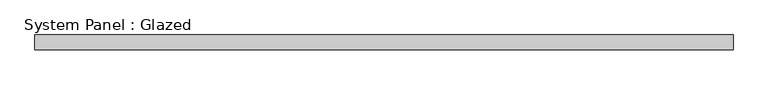
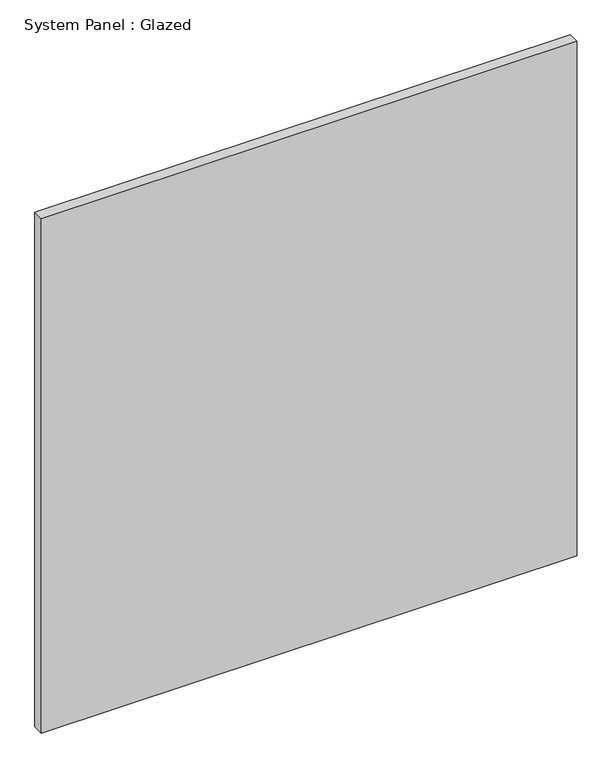
"""IFC4 building model written with IfcOpenShell, lengths in millimetres: plate geometry, System Panel : Glazed."""

from ifc_helpers import new_model, si_unit, origin, origin_with_axes, place, context, project, spatial, polyline, outline, extrude, source, transform, mapped, element, save


def system_panel_glazed_fe6f5f94(model_context):
    return source(origin(), model_context, "Body", "SweptSolid", [
        extrude(outline(polyline([(600.5514963, 19.05), (-600.5514963, 19.05), (-600.5514963, 44.45), (600.5514963, 44.45), (600.5514963, 19.05)])), origin_with_axes(), (0.0, 0.0, 1.0), 1219.2),
    ])


if __name__ == "__main__":
    model = new_model("IFC4")
    model_context = context("Model", 3, world=origin())
    ifc_project = project(units=[si_unit("LENGTHUNIT", "METRE", prefix="MILLI")], contexts=[model_context])
    site = spatial("IfcSite", under=ifc_project)
    building = spatial("IfcBuilding", under=site)
    placement = place(None, origin())
    system_panel_glazed_shape = system_panel_glazed_fe6f5f94(model_context)
    element("IfcPlate", 1, ObjectType="System Panel : Glazed", at=placement, inside=building, context=model_context, shape_type="MappedRepresentation", body=[
        mapped(system_panel_glazed_shape, transform((0.0, 0.0, 0.0), x_axis=(1.0, 0.0, 0.0), y_axis=(0.0, 1.0, 0.0), z_axis=(0.0, 0.0, 1.0))),
    ])
    save(model, "model.ifc")

# Revit data of these elements
# Type "System Panel : Glazed"
#   Construction Type Id = "GSP4R"
#   Analytic Construction = "1/8 in Pilkington single glazing"
#   Visual Light Transmittance = 0.9
#   Solar Heat Gain Coefficient = 0.86
#   Heat Transfer Coefficient (U) = 1.18115 BTU/(h·ft²·°F)
# Element 1 (IfcPlate, "System Panel : Glazed")
#   Materials on its faces: "Glass"
# Materials
#   "Glass": class "Glass", colour RGB 0 128 192, transparency 0.75, Description = "Soda Lime Glass", Cost = 0
